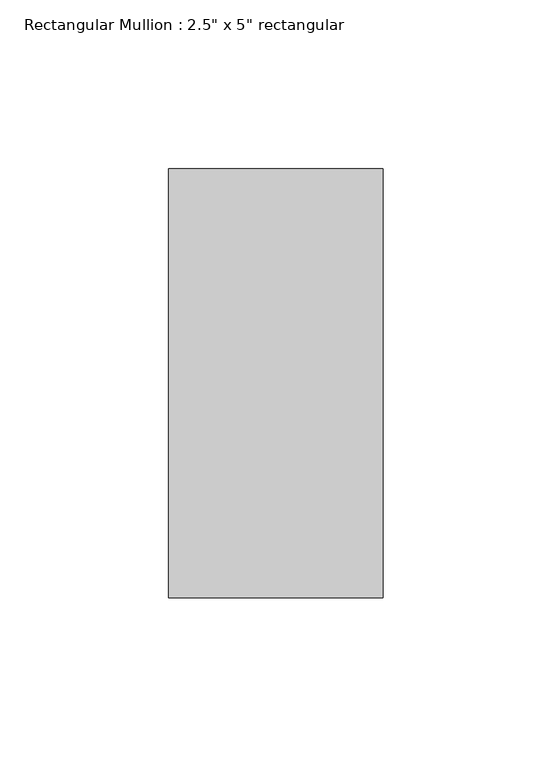
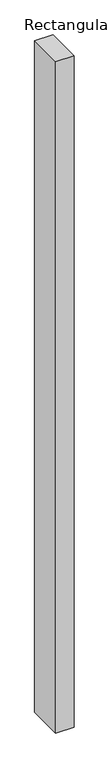
"""IFC4 building model written with IfcOpenShell, lengths in millimetres: member geometry."""

from ifc_helpers import new_model, si_unit, frame, origin, place, context, project, spatial, polyline, outline, extrude, source, transform, mapped, element, save


def member_029677a6(model_context):
    return source(origin(), model_context, "Body", "SweptSolid", [
        extrude(outline(polyline([(0.0, 63.5), (0.0, -63.5), (-63.5, -63.5), (-63.5, 63.5), (0.0, 63.5)])), frame((0.0, 0.0, -2477.2224322), z_axis=(0.0, 0.0, 1.0), x_axis=(1.0, 0.0, 0.0)), (0.0, 0.0, 1.0), 2477.2224322),
    ])


if __name__ == "__main__":
    model = new_model("IFC4")
    model_context = context("Model", 3, world=origin())
    ifc_project = project(units=[si_unit("LENGTHUNIT", "METRE", prefix="MILLI")], contexts=[model_context])
    site = spatial("IfcSite", under=ifc_project)
    building = spatial("IfcBuilding", under=site)
    placement = place(None, origin())
    member_shape = member_029677a6(model_context)
    element("IfcMember", 1, ObjectType="Rectangular Mullion : 2.5\" x 5\" rectangular", at=placement, inside=building, context=model_context, shape_type="MappedRepresentation", body=[
        mapped(member_shape, transform((0.0, 0.0, 0.0), x_axis=(1.0, 0.0, 0.0), y_axis=(0.0, 1.0, 0.0), z_axis=(0.0, 0.0, 1.0))),
    ])
    save(model, "model.ifc")

# Revit data of these elements
# Type "Rectangular Mullion : 2.5\" x 5\" rectangular"
#   built-in parameter 1007304 = 0.416667 (stored number, unit not read)
#   built-in parameter 1007301 = 0.104167 (stored number, unit not read)
#   built-in parameter 1007300 = 0.104167 (stored number, unit not read)
# Element 1 (IfcMember, "Rectangular Mullion : 2.5\" x 5\" rectangular")
#   Materials on its faces: "Aluminum"
# Materials
#   "Aluminum": class "Metal", colour RGB 247 247 247, transparency 0, Description = "Aluminum 6061", Cost = 0
